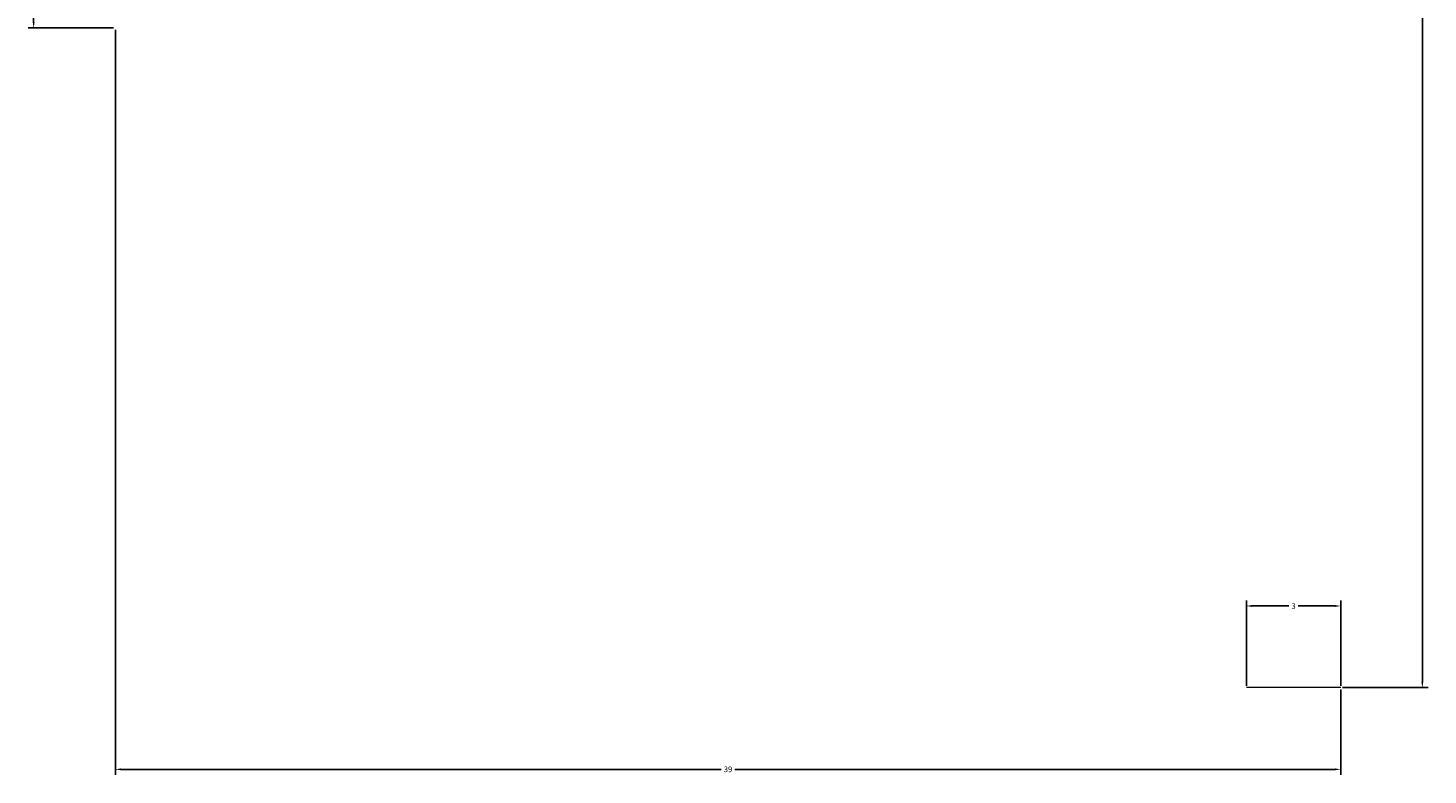
# Model space of a CAD drawing. Units: millimetres. Extents: x 3.7 to 48.2, y -50.7 to 2.9.
# Tile 1 of 2: x 3.7 to 48.2, y -50.7 to -26.9. Entities that reach past the tile are written whole.
import ezdxf

# ---------------------------------------------------------------- set-up
doc = ezdxf.new("R2010")
doc.units = ezdxf.units.MM
doc.header["$MEASUREMENT"] = 0
doc.layers.add('M-CONS', color=8, linetype='Continuous', lineweight=18)
doc.layers.add('M-DIMS', color=2, linetype='Continuous', lineweight=18)
doc.styles.get("Standard").update_dxf_attribs({"font": 'arial.ttf'})
doc.dimstyles.get("Standard").update_dxf_attribs({"dimtxt": 0.18, "dimasz": 0.18, "dimexe": 0.18, "dimexo": 0.0625, "dimgap": 0.09, "dimtad": 0, "dimtih": 1, "dimtoh": 1, "dimdec": 4, "dimzin": 0, "dimdsep": 46, "dimtxsty": 'Standard', "dimcen": 0.09, "dimadec": 0, "dimazin": 0, "dimtfac": 1, "dimtdec": 4, "dimtofl": 0, "dimtmove": 0, "dimatfit": 3, "dimfxl": 1, "dimtolj": 1, "dimtzin": 0, "dimarcsym": 0})

# ---------------------------------------------------------------- blocks, each defined once
blk = doc.blocks.new('*D3')
at = {"layer": 'Defpoints', "color": 0, "transparency": 16777216}
for p in [(6.456, -26.906), (45.456, -47.906), (45.456, -50.506)]:
    blk.add_point(p, dxfattribs=at)
at = {"layer": 'M-DIMS', "color": 0, "lineweight": -2, "transparency": 16777216}
for p, q in [((6.456, -26.969), (6.456, -50.686)), ((45.456, -47.969), (45.456, -50.686)), ((6.636, -50.506), (25.737, -50.506)), ((45.276, -50.506), (26.175, -50.506))]:
    blk.add_line(p, q, dxfattribs=at)
at = {"layer": 'M-DIMS', "color": 0, "transparency": 16777216}
for points in [[(6.636, -50.476), (6.636, -50.536), (6.456, -50.506)], [(45.276, -50.476), (45.276, -50.536), (45.456, -50.506)]]:
    blk.add_solid(points, dxfattribs=at)
at = {"layer": 'M-DIMS', "color": 0, "transparency": 16777216, "insert": (25.956, -50.506), "char_height": 0.18, "attachment_point": 5}
blk.add_mtext('\\A1;39', dxfattribs=at)
blk = doc.blocks.new('*D4')
at = {"layer": 'Defpoints', "color": 0, "transparency": 16777216}
for p in [(36.456, 0.094), (45.456, -47.906), (48.056, -47.906)]:
    blk.add_point(p, dxfattribs=at)
at = {"layer": 'M-DIMS', "color": 0, "lineweight": -2, "transparency": 16777216}
for p, q in [((36.518, 0.094), (48.236, 0.094)), ((48.056, -0.086), (48.056, -23.724)), ((48.056, -47.726), (48.056, -24.088)), ((45.518, -47.906), (48.236, -47.906))]:
    blk.add_line(p, q, dxfattribs=at)
at = {"layer": 'M-DIMS', "color": 0, "transparency": 16777216}
for points in [[(48.026, -0.086), (48.086, -0.086), (48.056, 0.094)], [(48.026, -47.726), (48.086, -47.726), (48.056, -47.906)]]:
    blk.add_solid(points, dxfattribs=at)
at = {"layer": 'M-DIMS', "color": 0, "transparency": 16777216, "insert": (48.056, -23.906), "char_height": 0.18, "attachment_point": 5}
blk.add_mtext('\\A1;48', dxfattribs=at)
blk = doc.blocks.new('*D6')
at = {"layer": 'Defpoints', "color": 0, "transparency": 16777216}
for p in [(3.856, -20.906), (6.456, -20.906), (6.456, -26.906)]:
    blk.add_point(p, dxfattribs=at)
at = {"layer": 'M-DIMS', "color": 0, "lineweight": -2, "transparency": 16777216}
for p, q in [((6.393, -20.906), (3.676, -20.906)), ((3.856, -21.086), (3.856, -23.724)), ((3.856, -26.726), (3.856, -24.088)), ((6.393, -26.906), (3.676, -26.906))]:
    blk.add_line(p, q, dxfattribs=at)
at = {"layer": 'M-DIMS', "color": 0, "transparency": 16777216}
for points in [[(3.826, -21.086), (3.886, -21.086), (3.856, -20.906)], [(3.826, -26.726), (3.886, -26.726), (3.856, -26.906)]]:
    blk.add_solid(points, dxfattribs=at)
at = {"layer": 'M-DIMS', "color": 0, "transparency": 16777216, "insert": (3.856, -23.906), "char_height": 0.18, "attachment_point": 5}
blk.add_mtext('\\A1;6', dxfattribs=at)
blk = doc.blocks.new('*D8')
at = {"layer": 'Defpoints', "color": 0, "transparency": 16777216}
for p in [(45.456, -45.306), (42.456, -47.906), (45.456, -47.906)]:
    blk.add_point(p, dxfattribs=at)
at = {"layer": 'M-DIMS', "color": 0, "lineweight": -2, "transparency": 16777216}
for p, q in [((42.456, -47.844), (42.456, -45.126)), ((42.636, -45.306), (43.807, -45.306)), ((45.276, -45.306), (44.105, -45.306)), ((45.456, -47.844), (45.456, -45.126))]:
    blk.add_line(p, q, dxfattribs=at)
at = {"layer": 'M-DIMS', "color": 0, "transparency": 16777216}
for points in [[(42.636, -45.276), (42.636, -45.336), (42.456, -45.306)], [(45.276, -45.276), (45.276, -45.336), (45.456, -45.306)]]:
    blk.add_solid(points, dxfattribs=at)
at = {"layer": 'M-DIMS', "color": 0, "transparency": 16777216, "insert": (43.956, -45.306), "char_height": 0.18, "attachment_point": 5}
blk.add_mtext('\\A1;3', dxfattribs=at)

msp = doc.modelspace()

# ---------------------------------------------------------------- linework, layer by layer
at = {"layer": 'M-CONS'}
msp.add_line((45.456, -47.906, 9), (42.456, -47.906, 9), dxfattribs=at)

# ---------------------------------------------------------------- dimensions: what is measured, and where the dimension line sits
at = {"layer": 'M-DIMS'}
for base, p1, p2, picture, middle in [((48.056, -47.906), (36.456, 0.094), (45.456, -47.906), '*D4', (48.056, -23.906)), ((3.856, -20.906), (6.456, -26.906), (6.456, -20.906), '*D6', (3.856, -23.906))]:
    dim = msp.add_linear_dim(base=base, p1=p1, p2=p2, angle=90, dimstyle='Standard', override={"dimdec": 0, "dimlfac": 1, "dimrnd": 0, "dimzin": 0, "dimdsep": 46, "dimlunit": 2}, dxfattribs=at)
    dim.commit()
    dim.dimension.update_dxf_attribs({"geometry": picture, "text_midpoint": middle})
for base, p1, picture, middle in [((45.456, -50.506), (6.456, -26.906), '*D3', (25.956, -50.506)), ((45.456, -45.306), (42.456, -47.906), '*D8', (43.956, -45.306))]:
    dim = msp.add_linear_dim(base=base, p1=p1, p2=(45.456, -47.906), dimstyle='Standard', override={"dimdec": 0, "dimlfac": 1, "dimrnd": 0, "dimzin": 0, "dimdsep": 46, "dimlunit": 2}, dxfattribs=at)
    dim.commit()
    dim.dimension.update_dxf_attribs({"geometry": picture, "text_midpoint": middle})

doc.saveas('drawing.dxf')
